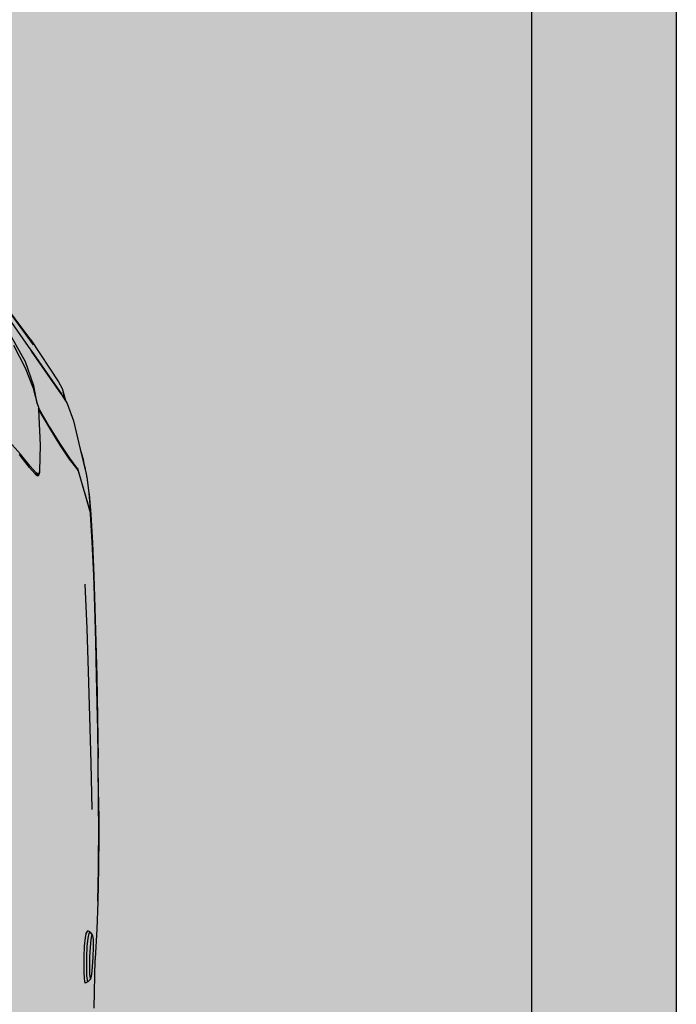
# Model space of a CAD drawing. Units: inches. Extents: x 1884 to 2398, y 474 to 1488.
# Tile 30 of 39: x 2356 to 2397, y 699 to 761. Entities that reach past the tile are written whole.
import ezdxf

# ---------------------------------------------------------------- set-up
doc = ezdxf.new("R2010")
doc.units = ezdxf.units.IN
doc.header["$MEASUREMENT"] = 0
doc.layers.get('0').update_dxf_attribs({"color": 250})
for name, color, linetype, lineweight in [('A-ANNO-DIMS', 2, 'Continuous', 18), ('A-WALL-PATT', 250, 'Continuous', 13), ('C-PROP', 7, 'Continuous', 30), ('C-VEHI', 8, 'Continuous', 18)]:
    doc.layers.add(name, color=color, linetype=linetype, lineweight=lineweight)
doc.layers.add('Edges', color=250, linetype='Continuous')
doc.layers.add('L-PVMT-PATT', color=9, linetype='Continuous', lineweight=13, true_color=0xc7c8ca)
doc.styles.get("Standard").update_dxf_attribs({"font": 'arial.ttf'})
doc.dimstyles.get("Standard").update_dxf_attribs({"dimtxt": 7, "dimasz": 0.18, "dimexe": 0.18, "dimexo": 0.0625, "dimgap": 0.09, "dimtad": 0, "dimtih": 1, "dimtoh": 1, "dimzin": 0, "dimdsep": 46, "dimlunit": 3, "dimtxsty": 'Standard', "dimcen": 0.09, "dimadec": 0, "dimazin": 0, "dimtfac": 1, "dimtofl": 0, "dimtmove": 0, "dimatfit": 3, "dimfxl": 1, "dimtolj": 1, "dimtzin": 0, "dimarcsym": 0})

# ---------------------------------------------------------------- blocks, each defined once
blk = doc.blocks.new('Nissan Qashqai pl')
at = {"layer": 'Edges'}
for p, q in [((7.9137, 12.815), (7.869, 12.8124)), ((7.87, 12.8126), (7.9151, 12.8152)), ((7.9658, 12.8172), (7.9137, 12.815)), ((7.9151, 12.8152), (7.9668, 12.8174)), ((8.016, 12.8189), (7.9658, 12.8172)), ((7.9668, 12.8174), (8.0168, 12.8191)), ((8.0713, 12.8205), (8.016, 12.8189)), ((8.0168, 12.8191), (8.0718, 12.8207)), ((8.1249, 12.8218), (8.0713, 12.8205)), ((8.0718, 12.8207), (8.1251, 12.822)), ((8.1901, 12.8232), (8.1249, 12.8218)), ((8.1251, 12.822), (8.1902, 12.8233)), ((8.2094, 12.8235), (8.1901, 12.8232)), ((8.1902, 12.8233), (8.2543, 12.8243)), ((8.2543, 12.8243), (8.2094, 12.8235)), ((8.2543, 12.8243), (8.2094, 12.8235)), ((8.2544, 12.8242), (8.2094, 12.8235)), ((8.2693, 12.8245), (8.2543, 12.8243)), ((8.3166, 12.8249), (8.2544, 12.8242)), ((8.2622, 12.8125), (8.3356, 12.8141)), ((8.3098, 12.825), (8.2693, 12.8245)), ((8.3159, 12.825), (8.2693, 12.8245)), ((8.3159, 12.825), (8.3098, 12.825)), ((8.3159, 12.825), (8.3163, 12.825)), ((8.3163, 12.825), (8.3657, 12.8252)), ((8.3163, 12.825), (8.3597, 12.8252)), ((8.3764, 12.8251), (8.3166, 12.8249)), ((8.3597, 12.8252), (8.3657, 12.8252)), ((8.3657, 12.8252), (8.3663, 12.8252)), ((8.3663, 12.8252), (8.3747, 12.8252)), ((8.3764, 12.8251), (8.3663, 12.8252)), ((8.3747, 12.8252), (8.3757, 12.8252)), ((8.3757, 12.8252), (8.4282, 12.8249)), ((8.4069, 12.8249), (8.3764, 12.8251)), ((8.4219, 12.8246), (8.4069, 12.8249)), ((8.4292, 12.8248), (8.4069, 12.8249)), ((8.4282, 12.8249), (8.4799, 12.8239)), ((8.4799, 12.8239), (8.4292, 12.8248)), ((8.4799, 12.8239), (8.4811, 12.8239)), ((8.4811, 12.8239), (8.5241, 12.8222)), ((8.5241, 12.8222), (8.5707, 12.8193)), ((8.5287, 12.8112), (8.5331, 12.815)), ((8.5347, 12.8159), (8.5331, 12.815)), ((8.5331, 12.815), (8.5346, 12.8138)), ((8.5346, 12.8138), (8.5406, 12.8125)), ((8.5407, 12.8167), (8.5347, 12.8159)), ((8.5527, 12.8169), (8.5407, 12.8167)), ((8.5682, 12.8164), (8.5527, 12.8169)), ((8.5837, 12.8154), (8.5682, 12.8164)), ((8.5707, 12.8193), (8.5719, 12.8193)), ((8.6489, 12.8179), (8.5719, 12.8193)), ((8.5958, 12.8141), (8.5837, 12.8154)), ((8.6018, 12.8129), (8.5958, 12.8141)), ((7.7673, 12.7961), (7.8058, 12.8055)), ((7.7673, 12.7961), (7.7848, 12.8012)), ((7.7835, 12.8007), (7.7835, 12.8007)), ((7.8087, 12.8062), (7.7848, 12.8012)), ((7.7865, 12.8013), (7.7866, 12.8013)), ((7.7936, 12.8029), (7.7977, 12.8038)), ((7.8676, 12.8123), (7.7998, 12.7928)), ((7.8012, 12.7929), (7.8681, 12.8121)), ((7.8106, 12.8065), (7.8087, 12.8062)), ((7.8106, 12.8065), (7.8107, 12.8065)), ((7.8107, 12.8065), (7.8363, 12.8097)), ((7.8363, 12.8097), (7.8676, 12.8123)), ((7.8363, 12.8097), (7.8381, 12.81)), ((7.8381, 12.81), (7.87, 12.8126)), ((7.8676, 12.8123), (7.8681, 12.8121)), ((7.869, 12.8124), (7.8681, 12.8121)), ((7.9803, 12.803), (8.05, 12.8066)), ((8.05, 12.8066), (8.1176, 12.8087)), ((8.1176, 12.8087), (8.1888, 12.8107)), ((8.1888, 12.8107), (8.2622, 12.8125)), ((8.5287, 12.8112), (8.5269, 12.8082)), ((8.5322, 12.8047), (8.5269, 12.8082)), ((8.5287, 12.8112), (8.531, 12.8095)), ((8.531, 12.8095), (8.5385, 12.8079)), ((8.5322, 12.8047), (8.5375, 12.8036)), ((8.5375, 12.8036), (8.5513, 12.8023)), ((8.5385, 12.8079), (8.5518, 12.8066)), ((8.5406, 12.8125), (8.5526, 12.8114)), ((8.5513, 12.8023), (8.5678, 12.8016)), ((8.5518, 12.8066), (8.568, 12.8059)), ((8.5526, 12.8114), (8.5681, 12.8107)), ((8.5678, 12.8016), (8.5844, 12.8014)), ((8.568, 12.8059), (8.5842, 12.8057)), ((8.5681, 12.8107), (8.5836, 12.8104)), ((8.5836, 12.8104), (8.5957, 12.8107)), ((8.5842, 12.8057), (8.5974, 12.8061)), ((8.5844, 12.8014), (8.5921, 12.8016)), ((8.5921, 12.8016), (8.6021, 12.8022)), ((8.5957, 12.8107), (8.6017, 12.8114)), ((8.5974, 12.8061), (8.6049, 12.8069)), ((8.6017, 12.8114), (8.6032, 12.8121)), ((8.6032, 12.8121), (8.6018, 12.8129)), ((8.6021, 12.8022), (8.6065, 12.8027)), ((8.6073, 12.808), (8.6032, 12.8121)), ((8.6049, 12.8069), (8.6073, 12.808)), ((8.6065, 12.8027), (8.6093, 12.804)), ((8.6073, 12.808), (8.6093, 12.804)), ((7.6953, 12.7753), (7.7223, 12.7851)), ((7.7223, 12.7851), (7.7673, 12.7961)), ((7.7814, 12.7791), (7.7991, 12.7923)), ((7.7984, 12.7909), (7.7828, 12.7793)), ((7.7976, 12.792), (7.7991, 12.7923)), ((7.8007, 12.7926), (7.7984, 12.7909)), ((7.7991, 12.7923), (7.7998, 12.7928)), ((7.7995, 12.7924), (7.8007, 12.7926)), ((7.8012, 12.7929), (7.8007, 12.7926)), ((7.6608, 12.7617), (7.6712, 12.7675)), ((7.6712, 12.7675), (7.6721, 12.7679)), ((7.6926, 12.7737), (7.6721, 12.7679)), ((7.6911, 12.7728), (7.6774, 12.7688)), ((7.6802, 12.766), (7.6809, 12.7664)), ((7.6809, 12.7664), (7.6911, 12.7728)), ((7.6911, 12.7728), (7.6926, 12.7737)), ((7.6926, 12.7737), (7.6953, 12.7753)), ((7.7591, 12.7641), (7.7814, 12.7791)), ((7.7828, 12.7793), (7.7606, 12.7644)), ((7.5946, 12.718), (7.6608, 12.7617)), ((7.6113, 12.7186), (7.6759, 12.7633)), ((7.6799, 12.7658), (7.6125, 12.719)), ((7.6759, 12.7633), (7.6793, 12.7657)), ((7.6793, 12.7657), (7.6802, 12.766)), ((7.6799, 12.7658), (7.6802, 12.766)), ((7.7325, 12.7476), (7.7591, 12.7641)), ((7.7606, 12.7644), (7.7341, 12.7478)), ((7.7038, 12.731), (7.7325, 12.7476)), ((7.7341, 12.7478), (7.7056, 12.7314)), ((7.6024, 12.7221), (7.5387, 12.6759)), ((7.667, 12.723), (7.6295, 12.7097)), ((7.6386, 12.7089), (7.6708, 12.7217)), ((7.6949, 12.7283), (7.667, 12.723)), ((7.6708, 12.7217), (7.6949, 12.7283)), ((7.6949, 12.7283), (7.701, 12.73)), ((7.701, 12.73), (7.7024, 12.7301)), ((7.7024, 12.7301), (7.7038, 12.731)), ((7.7024, 12.7301), (7.7034, 12.7301)), ((7.7056, 12.7314), (7.7034, 12.7301)), ((7.7034, 12.7301), (7.7048, 12.7302)), ((7.7048, 12.7302), (7.7608, 12.7329)), ((7.7058, 12.7308), (7.7048, 12.7302)), ((7.7608, 12.7329), (7.8014, 12.7318)), ((7.7688, 12.7328), (7.7688, 12.734)), ((7.8045, 12.7263), (7.7938, 12.7171)), ((7.8062, 12.725), (7.7959, 12.7161)), ((7.8014, 12.7318), (7.8022, 12.7316)), ((7.8022, 12.7316), (7.8037, 12.7315)), ((7.8022, 12.7316), (7.8072, 12.73)), ((7.8037, 12.7315), (7.8096, 12.7294)), ((7.8072, 12.73), (7.8045, 12.7263)), ((7.8062, 12.725), (7.8087, 12.7283)), ((7.8066, 12.7254), (7.8062, 12.725)), ((7.8096, 12.7294), (7.8066, 12.7254)), ((7.8072, 12.73), (7.8087, 12.7283)), ((7.5946, 12.718), (7.5304, 12.6704)), ((7.5501, 12.6757), (7.6051, 12.7139)), ((7.6295, 12.7097), (7.59, 12.6877)), ((7.6032, 12.6908), (7.6386, 12.7089)), ((7.6051, 12.7139), (7.6113, 12.7186)), ((7.6051, 12.7139), (7.6111, 12.7181)), ((7.6118, 12.7186), (7.6111, 12.7181)), ((7.6125, 12.719), (7.6118, 12.7186)), ((7.7938, 12.7171), (7.7748, 12.7018)), ((7.7959, 12.7161), (7.7772, 12.7011)), ((7.7748, 12.7018), (7.7507, 12.6803)), ((7.7772, 12.7011), (7.776, 12.6999))]:
    blk.add_line(p, q, dxfattribs=at)
blk = doc.blocks.new('car')
blk.add_blockref('Nissan Qashqai pl', (-9.7433, -11.9151))
blk = doc.blocks.new('carr')
blk.add_blockref('car', (0.5124, -0.007))
blk = doc.blocks.new('*D49')
at = {"layer": 'A-ANNO-DIMS', "color": 0, "lineweight": -2, "transparency": 16777216}
for p, q in [((2318.409, 987.716), (2318.409, 484.005)), ((2340.409, 987.716), (2340.409, 484.005)), ((2318.589, 484.185), (2340.229, 484.185)), ((2340.409, 484.185), (2340.589, 484.185))]:
    blk.add_line(p, q, dxfattribs=at)
at = {"layer": 'A-ANNO-DIMS', "color": 0, "lineweight": 100, "transparency": 16777216}
for points in [[(2318.589, 484.215), (2318.589, 484.155), (2318.409, 484.185)], [(2340.229, 484.215), (2340.229, 484.155), (2340.409, 484.185)]]:
    blk.add_solid(points, dxfattribs=at)
at = {"layer": 'Defpoints', "color": 0, "lineweight": 100, "transparency": 16777216}
for p in [(2318.409, 987.778), (2340.409, 987.778), (2340.409, 484.185)]:
    blk.add_point(p, dxfattribs=at)
at = {"layer": 'A-ANNO-DIMS', "color": 0, "transparency": 16777216, "insert": (2352.373, 484.185), "char_height": 7, "attachment_point": 5}
blk.add_mtext('\\A1;1\'-10"', dxfattribs=at)

msp = doc.modelspace()

# ---------------------------------------------------------------- hatches: boundary and pattern name
at = {"layer": 'A-WALL-PATT'}
h = msp.add_hatch(color=256, dxfattribs=at)
h.dxf.hatch_style = 1
h.paths.add_polyline_path([(2351.529, 837.963), (2342.529, 837.963), (2342.529, 813.478), (2351.529, 813.478)])
h.paths.add_polyline_path([(2351.529, 782.175), (2342.529, 782.175), (2342.529, 778.966), (2238.447, 778.966), (2238.447, 769.966), (2351.529, 769.966)])
h.paths.add_polyline_path([(2351.529, 914.773), (2342.529, 914.773), (2342.529, 901.966), (2222.529, 901.966), (2222.529, 908.236), (2213.529, 908.236), (2213.529, 901.966), (2198.529, 901.966), (2198.529, 892.966), (2198.529, 815.857), (2203.029, 815.857), (2203.029, 892.966), (2342.529, 892.966), (2342.529, 869.555), (2346.047, 869.555), (2351.529, 869.555), (2351.529, 880.385)])
h.paths.add_polyline_path([(2208.948, 778.966), (2203.029, 778.966), (2203.029, 782.647), (2198.529, 782.647), (2198.529, 779.109), (2193.526, 779.109), (2193.526, 769.966), (2198.529, 769.966), (2208.948, 769.966)])
h.paths.add_polyline_path([(2126.529, 815.801), (2117.529, 815.801), (2117.529, 676.183), (2126.529, 676.183), (2126.529, 769.966), (2132.515, 769.966), (2132.515, 778.664), (2126.529, 778.664)])
h.paths.add_polyline_path([(2135.996, 901.385), (2009.529, 901.385), (2009.529, 929.544), (2000.529, 929.544), (2000.529, 892.385), (2117.529, 892.385), (2117.529, 880.382), (2126.529, 880.382), (2126.529, 892.385), (2135.996, 892.385)])
h.paths.add_polyline_path([(2198.529, 901.385), (2185.2, 901.385), (2185.2, 892.385), (2198.529, 892.385), (2198.529, 892.966)])
h.paths.add_polyline_path([(1961.529, 892.385), (1965.143, 892.385), (1965.143, 901.385), (1952.529, 901.385), (1952.529, 604.13), (1961.529, 604.13), (1961.529, 631.385), (1988.002, 631.385), (1988.002, 640.385), (1961.529, 640.385)])
h.paths.add_polyline_path([(1955.529, 604.13), (1952.529, 604.13), (1952.529, 530.885), (2126.529, 530.885), (2126.529, 533.885), (1955.529, 533.885)])
h.paths.add_polyline_path([(2396.529, 604.13), (2393.529, 604.13), (2393.529, 533.885), (2126.529, 533.885), (2126.529, 530.885), (2396.529, 530.885)])
h.paths.add_polyline_path([(2396.529, 779.322), (2387.529, 779.322), (2387.529, 604.13), (2396.529, 604.13)])
at = {"layer": 'L-PVMT-PATT'}
h = msp.add_hatch(color=256, dxfattribs=at)
h.dxf.hatch_style = 1
h.paths.add_polyline_path([(2387.529, 769.966), (2351.529, 769.966), (2238.447, 769.966), (2238.447, 762.15), (2238.447, 754.445), (2126.529, 754.445), (2126.529, 676.183), (2134.868, 676.183), (2142.673, 676.183), (2142.673, 646.578), (2134.868, 646.578), (2126.529, 646.578), (2126.529, 640.17), (2387.529, 640.17)])
h.paths.add_polyline_path([(2387.529, 631.385), (2303.086, 631.385), (2303.086, 615.671), (2387.529, 615.671)])
h.paths.add_polyline_path([(2387.529, 640.17), (2126.529, 640.17), (2126.529, 631.385), (2387.529, 631.385)])
h.paths.add_polyline_path([(2393.529, 604.13), (2387.529, 604.13), (2387.529, 615.671), (2303.086, 615.671), (2303.086, 607.943), (2249.649, 607.943), (2126.529, 607.943), (2126.529, 533.885), (2393.529, 533.885)])
h.paths.add_polyline_path([(2257.825, 611.008), (2257.83, 611.337), (2257.915, 616.493), (2258.021, 621.805), (2258.146, 627.274), (2258.252, 631.385), (2126.529, 631.385), (2126.529, 611.008)])
h.paths.add_polyline_path([(2258.892, 611.285), (2258.888, 611.008), (2300.247, 611.008), (2300.247, 631.385), (2259.314, 631.385), (2259.206, 627.173), (2259.081, 621.72), (2258.976, 616.424)])

# ---------------------------------------------------------------- linework, layer by layer
at = {"layer": 'C-PROP'}
for p, q in [((2396.529, 1406.885), (2396.529, 530.885)), ((2387.529, 779.322), (2387.529, 604.13))]:
    msp.add_line(p, q, dxfattribs=at)

# ---------------------------------------------------------------- block references
at = {"layer": 'C-VEHI', "xscale": 39.37007874015748, "yscale": 39.37007874015748, "zscale": 39.37007874015748, "rotation": 270}
msp.add_blockref('carr', (2325.111, 676.232), dxfattribs=at)

# ---------------------------------------------------------------- dimensions: what is measured, and where the dimension line sits
at = {"layer": 'A-ANNO-DIMS'}
dim = msp.add_linear_dim(base=(2340.409, 484.185), p1=(2318.409, 987.778), p2=(2340.409, 987.778), dimstyle='Standard', override={"dimdec": 1, "dimlfac": 1, "dimrnd": 0, "dimzin": 1, "dimdsep": 46, "dimlunit": 4, "dimfrac": 2}, dxfattribs=at)
dim.commit()
dim.dimension.update_dxf_attribs({"geometry": '*D49', "text_midpoint": (2352.373, 484.185)})

doc.saveas('drawing.dxf')
